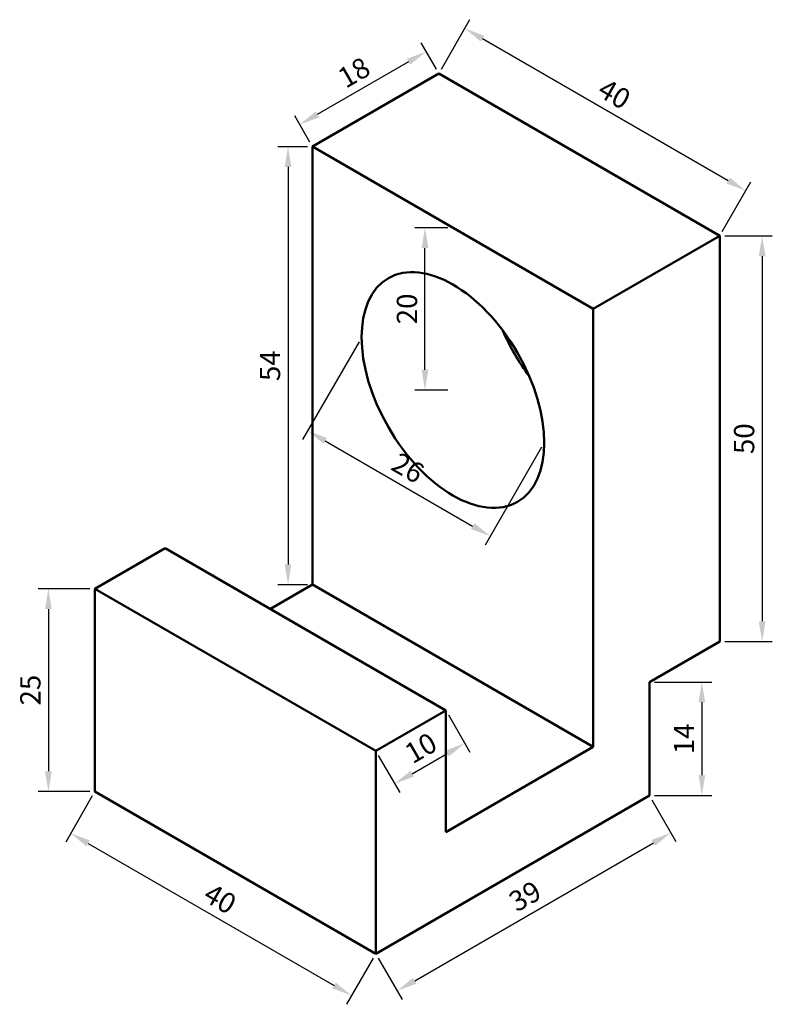
# Model space of a CAD drawing. Units: millimetres. Extents: x 3000 to 3093, y 728 to 849.
import ezdxf

# ---------------------------------------------------------------- set-up
doc = ezdxf.new("R2010")
doc.units = ezdxf.units.MM
doc.layers.add('M-DIMS', color=2, linetype='Continuous', lineweight=25)
doc.layers.add('M-OUTL', color=7, linetype='Continuous', lineweight=50)
doc.styles.get("Standard").update_dxf_attribs({"font": 'arial.ttf'})
doc.dimstyles.new('ISO-25', dxfattribs={"dimtxt": 2.5, "dimasz": 2.5, "dimexe": 1.25, "dimexo": 0.625, "dimtad": 1, "dimtxsty": 'Standard', "dimcen": 2.5, "dimadec": 0, "dimazin": 0, "dimtfac": 1, "dimtmove": 0, "dimatfit": 3, "dimfxl": 1, "dimarcsym": 0})

# ---------------------------------------------------------------- blocks, each defined once
blk = doc.blocks.new('*D1')
at = {"layer": 'Defpoints', "color": 0, "transparency": 16777216}
for p in [(3051.81, 842.52), (3089.67, 828.09), (3086.45, 822.52)]:
    blk.add_point(p, dxfattribs=at)
at = {"layer": 'M-DIMS', "color": 0, "lineweight": -2, "transparency": 16777216}
for p, q in [((3052.12, 843.06), (3055.65, 849.18)), ((3057.19, 846.84), (3087.5, 829.34)), ((3086.76, 823.06), (3090.29, 829.18))]:
    blk.add_line(p, q, dxfattribs=at)
at = {"layer": 'M-DIMS', "color": 0, "transparency": 16777216}
for points in [[(3057.4, 847.2), (3056.98, 846.48), (3055.03, 848.09)], [(3087.71, 829.7), (3087.3, 828.98), (3089.67, 828.09)]]:
    blk.add_solid(points, dxfattribs=at)
at = {"layer": 'M-DIMS', "color": 0, "transparency": 16777216, "insert": (3073.3, 839.74), "char_height": 2.5, "attachment_point": 5, "rotation": 330}
blk.add_mtext('40', dxfattribs=at)
blk = doc.blocks.new('*D2')
at = {"layer": 'Defpoints', "color": 0, "transparency": 16777216}
for p in [(3086.45, 822.52), (3086.45, 772.52), (3091.69, 772.52)]:
    blk.add_point(p, dxfattribs=at)
at = {"layer": 'M-DIMS', "color": 0, "lineweight": -2, "transparency": 16777216}
for p, q in [((3087.08, 822.52), (3092.94, 822.52)), ((3091.69, 820.02), (3091.69, 775.02)), ((3087.08, 772.52), (3092.94, 772.52))]:
    blk.add_line(p, q, dxfattribs=at)
at = {"layer": 'M-DIMS', "color": 0, "transparency": 16777216}
for points in [[(3091.27, 820.02), (3092.11, 820.02), (3091.69, 822.52)], [(3091.27, 775.02), (3092.11, 775.02), (3091.69, 772.52)]]:
    blk.add_solid(points, dxfattribs=at)
at = {"layer": 'M-DIMS', "color": 0, "transparency": 16777216, "insert": (3089.79, 797.52), "char_height": 2.5, "attachment_point": 5, "rotation": 90}
blk.add_mtext('50', dxfattribs=at)
blk = doc.blocks.new('*D3')
at = {"layer": 'Defpoints', "color": 0, "transparency": 16777216}
for p in [(3051.81, 842.52), (3034.65, 836.24), (3036.22, 833.52)]:
    blk.add_point(p, dxfattribs=at)
at = {"layer": 'M-DIMS', "color": 0, "lineweight": -2, "transparency": 16777216}
for p, q in [((3051.5, 843.06), (3049.62, 846.32)), ((3048.08, 843.99), (3036.82, 837.49)), ((3035.91, 834.06), (3034.03, 837.32))]:
    blk.add_line(p, q, dxfattribs=at)
at = {"layer": 'M-DIMS', "color": 0, "transparency": 16777216}
for points in [[(3047.87, 844.35), (3048.28, 843.63), (3050.24, 845.24)], [(3036.61, 837.85), (3037.03, 837.13), (3034.65, 836.24)]]:
    blk.add_solid(points, dxfattribs=at)
at = {"layer": 'M-DIMS', "color": 0, "transparency": 16777216, "insert": (3041.5, 842.39), "char_height": 2.5, "attachment_point": 5, "rotation": 30}
blk.add_mtext('18', dxfattribs=at)
blk = doc.blocks.new('*D4')
at = {"layer": 'Defpoints', "color": 0, "transparency": 16777216}
for p in [(3036.22, 833.52), (3033.21, 779.52), (3036.22, 779.52)]:
    blk.add_point(p, dxfattribs=at)
at = {"layer": 'M-DIMS', "color": 0, "lineweight": -2, "transparency": 16777216}
for p, q in [((3035.6, 833.52), (3031.96, 833.52)), ((3033.21, 831.02), (3033.21, 782.02)), ((3035.6, 779.52), (3031.96, 779.52))]:
    blk.add_line(p, q, dxfattribs=at)
at = {"layer": 'M-DIMS', "color": 0, "transparency": 16777216}
for points in [[(3032.79, 831.02), (3033.62, 831.02), (3033.21, 833.52)], [(3032.79, 782.02), (3033.62, 782.02), (3033.21, 779.52)]]:
    blk.add_solid(points, dxfattribs=at)
at = {"layer": 'M-DIMS', "color": 0, "transparency": 16777216, "insert": (3031.31, 806.52), "char_height": 2.5, "attachment_point": 5, "rotation": 90}
blk.add_mtext('54', dxfattribs=at)
blk = doc.blocks.new('*D5')
at = {"layer": 'Defpoints', "color": 0, "transparency": 16777216}
for p in [(3009.38, 779.02), (3003.65, 754.02), (3009.38, 754.02)]:
    blk.add_point(p, dxfattribs=at)
at = {"layer": 'M-DIMS', "color": 0, "lineweight": -2, "transparency": 16777216}
for p, q in [((3008.75, 779.02), (3002.4, 779.02)), ((3003.65, 776.52), (3003.65, 756.52)), ((3008.75, 754.02), (3002.4, 754.02))]:
    blk.add_line(p, q, dxfattribs=at)
at = {"layer": 'M-DIMS', "color": 0, "transparency": 16777216}
for points in [[(3003.23, 776.52), (3004.07, 776.52), (3003.65, 779.02)], [(3003.23, 756.52), (3004.07, 756.52), (3003.65, 754.02)]]:
    blk.add_solid(points, dxfattribs=at)
at = {"layer": 'M-DIMS', "color": 0, "transparency": 16777216, "insert": (3001.75, 766.52), "char_height": 2.5, "attachment_point": 5, "rotation": 90}
blk.add_mtext('25', dxfattribs=at)
blk = doc.blocks.new('*D6')
at = {"layer": 'Defpoints', "color": 0, "transparency": 16777216}
for p in [(3009.38, 754.02), (3044.02, 734.02), (3041.04, 728.87)]:
    blk.add_point(p, dxfattribs=at)
at = {"layer": 'M-DIMS', "color": 0, "lineweight": -2, "transparency": 16777216}
for p, q in [((3009.06, 753.48), (3005.78, 747.79)), ((3008.57, 747.62), (3038.88, 730.12)), ((3043.7, 733.48), (3040.42, 727.79))]:
    blk.add_line(p, q, dxfattribs=at)
at = {"layer": 'M-DIMS', "color": 0, "transparency": 16777216}
for points in [[(3008.77, 747.98), (3008.36, 747.26), (3006.4, 748.87)], [(3039.08, 730.48), (3038.67, 729.76), (3041.04, 728.87)]]:
    blk.add_solid(points, dxfattribs=at)
at = {"layer": 'M-DIMS', "color": 0, "transparency": 16777216, "insert": (3024.67, 740.52), "char_height": 2.5, "attachment_point": 5, "rotation": 330}
blk.add_mtext('40', dxfattribs=at)
blk = doc.blocks.new('*D7')
at = {"layer": 'Defpoints', "color": 0, "transparency": 16777216}
for p in [(3077.79, 753.52), (3080.44, 748.94), (3044.02, 734.02)]:
    blk.add_point(p, dxfattribs=at)
at = {"layer": 'M-DIMS', "color": 0, "lineweight": -2, "transparency": 16777216}
for p, q in [((3078.1, 752.98), (3081.06, 747.86)), ((3048.83, 730.69), (3078.27, 747.69)), ((3044.33, 733.48), (3047.29, 728.36))]:
    blk.add_line(p, q, dxfattribs=at)
at = {"layer": 'M-DIMS', "color": 0, "transparency": 16777216}
for points in [[(3078.06, 748.05), (3078.48, 747.33), (3080.44, 748.94)], [(3048.62, 731.05), (3049.04, 730.33), (3046.66, 729.44)]]:
    blk.add_solid(points, dxfattribs=at)
at = {"layer": 'M-DIMS', "color": 0, "transparency": 16777216, "insert": (3062.6, 740.84), "char_height": 2.5, "attachment_point": 5, "rotation": 30}
blk.add_mtext('39', dxfattribs=at)
blk = doc.blocks.new('*D8')
at = {"layer": 'Defpoints', "color": 0, "transparency": 16777216}
for p in [(3077.79, 767.52), (3077.79, 753.52), (3084.25, 753.52)]:
    blk.add_point(p, dxfattribs=at)
at = {"layer": 'M-DIMS', "color": 0, "lineweight": -2, "transparency": 16777216}
for p, q in [((3078.42, 767.52), (3085.5, 767.52)), ((3084.25, 765.02), (3084.25, 756.02)), ((3078.42, 753.52), (3085.5, 753.52))]:
    blk.add_line(p, q, dxfattribs=at)
at = {"layer": 'M-DIMS', "color": 0, "transparency": 16777216}
for points in [[(3083.84, 765.02), (3084.67, 765.02), (3084.25, 767.52)], [(3083.84, 756.02), (3084.67, 756.02), (3084.25, 753.52)]]:
    blk.add_solid(points, dxfattribs=at)
at = {"layer": 'M-DIMS', "color": 0, "transparency": 16777216, "insert": (3082.37, 760.52), "char_height": 2.5, "attachment_point": 5, "rotation": 90}
blk.add_mtext('14', dxfattribs=at)
blk = doc.blocks.new('*D9')
at = {"layer": 'Defpoints', "color": 0, "transparency": 16777216}
for p in [(3052.68, 764.02), (3055.02, 759.97), (3044.02, 759.02)]:
    blk.add_point(p, dxfattribs=at)
at = {"layer": 'M-DIMS', "color": 0, "lineweight": -2, "transparency": 16777216}
for p, q in [((3052.99, 763.48), (3055.64, 758.88)), ((3048.52, 756.22), (3052.85, 758.72)), ((3044.33, 758.48), (3046.98, 753.88))]:
    blk.add_line(p, q, dxfattribs=at)
at = {"layer": 'M-DIMS', "color": 0, "transparency": 16777216}
for points in [[(3052.65, 759.08), (3053.06, 758.36), (3055.02, 759.97)], [(3048.32, 756.58), (3048.73, 755.86), (3046.36, 754.97)]]:
    blk.add_solid(points, dxfattribs=at)
at = {"layer": 'M-DIMS', "color": 0, "transparency": 16777216, "insert": (3049.74, 759.11), "char_height": 2.5, "attachment_point": 5, "rotation": 30}
blk.add_mtext('10', dxfattribs=at)
blk = doc.blocks.new('*D10')
at = {"layer": 'Defpoints', "color": 0, "transparency": 16777216}
for p in [(3050.1, 823.52), (3053.54, 823.52), (3053.54, 803.52)]:
    blk.add_point(p, dxfattribs=at)
at = {"layer": 'M-DIMS', "color": 0, "lineweight": -2, "transparency": 16777216}
for p, q in [((3052.92, 823.52), (3048.85, 823.52)), ((3050.1, 806.02), (3050.1, 821.02)), ((3052.92, 803.52), (3048.85, 803.52))]:
    blk.add_line(p, q, dxfattribs=at)
at = {"layer": 'M-DIMS', "color": 0, "transparency": 16777216}
for points in [[(3049.69, 821.02), (3050.52, 821.02), (3050.1, 823.52)], [(3049.69, 806.02), (3050.52, 806.02), (3050.1, 803.52)]]:
    blk.add_solid(points, dxfattribs=at)
at = {"layer": 'M-DIMS', "color": 0, "transparency": 16777216, "insert": (3048.2, 813.52), "char_height": 2.5, "attachment_point": 5, "rotation": 90}
blk.add_mtext('20', dxfattribs=at)
blk = doc.blocks.new('*D11')
at = {"layer": 'Defpoints', "color": 0, "transparency": 16777216}
for p in [(3042.28, 810.02), (3064.8, 797.02), (3058.15, 785.5)]:
    blk.add_point(p, dxfattribs=at)
at = {"layer": 'M-DIMS', "color": 0, "lineweight": -2, "transparency": 16777216}
for p, q in [((3041.97, 809.48), (3035.01, 797.41)), ((3037.8, 797.25), (3055.98, 786.75)), ((3064.49, 796.48), (3057.52, 784.41))]:
    blk.add_line(p, q, dxfattribs=at)
at = {"layer": 'M-DIMS', "color": 0, "transparency": 16777216}
for points in [[(3038, 797.61), (3037.59, 796.89), (3035.63, 798.5)], [(3056.19, 787.11), (3055.77, 786.39), (3058.15, 785.5)]]:
    blk.add_solid(points, dxfattribs=at)
at = {"layer": 'M-DIMS', "color": 0, "transparency": 16777216, "insert": (3047.84, 793.64), "char_height": 2.5, "attachment_point": 5, "rotation": 330}
blk.add_mtext('26', dxfattribs=at)

msp = doc.modelspace()

# ---------------------------------------------------------------- linework, layer by layer
at = {"layer": 'M-OUTL'}
for p, q in [((3051.811, 842.522), (3036.223, 833.522)), ((3086.452, 822.522), (3051.811, 842.522)), ((3036.223, 833.522), (3070.864, 813.522)), ((3036.223, 833.522), (3036.223, 779.522)), ((3070.864, 813.522), (3086.452, 822.522)), ((3086.452, 772.522), (3086.452, 822.522)), ((3070.864, 813.522), (3070.864, 759.522)), ((3009.376, 779.022), (3018.036, 784.022)), ((3018.036, 784.022), (3052.677, 764.022)), ((3036.223, 779.522), (3031.027, 776.522)), ((3036.223, 779.522), (3070.864, 759.522)), ((3009.376, 754.022), (3009.376, 779.022)), ((3044.017, 759.022), (3009.376, 779.022)), ((3077.792, 767.522), (3086.452, 772.522)), ((3077.792, 753.522), (3077.792, 767.522)), ((3044.017, 759.022), (3052.677, 764.022)), ((3052.677, 749.022), (3052.677, 764.022)), ((3044.017, 759.022), (3044.017, 734.022)), ((3044.017, 734.022), (3044.017, 759.022)), ((3070.864, 759.522), (3052.677, 749.022)), ((3044.017, 734.022), (3009.376, 754.022)), ((3044.017, 734.022), (3077.792, 753.522))]:
    msp.add_line(p, q, dxfattribs=at)
msp.add_ellipse((3053.543, 803.522), major_axis=(7.961, -13.789), ratio=0.5773503, dxfattribs=at)
msp.add_ellipse((3069.132, 812.522), major_axis=(7.961, -13.789), ratio=0.5773503, start_param=4.5074378, end_param=4.9173401, dxfattribs=at)

# ---------------------------------------------------------------- dimensions: what is measured, and where the dimension line sits
at = {"layer": 'M-DIMS'}
for p1, p2, distance, picture, middle in [((3051.811, 842.522), (3086.452, 822.522), 6.432, '*D1', (3073.299, 839.74)), ((3051.811, 842.522), (3036.223, 833.522), -3.14, '*D3', (3041.496, 842.389)), ((3036.223, 833.522), (3036.223, 779.522), -3.015, '*D4', (3031.311, 806.522)), ((3053.543, 803.522), (3053.543, 823.522), 3.44, '*D10', (3048.202, 813.522)), ((3086.452, 822.522), (3086.452, 772.522), 5.239, '*D2', (3089.79, 797.522)), ((3042.285, 810.022), (3064.802, 797.022), -13.308, '*D11', (3047.84, 793.644)), ((3009.376, 779.022), (3009.376, 754.022), -5.726, '*D5', (3001.748, 766.522)), ((3077.792, 767.522), (3077.792, 753.522), 6.461, '*D8', (3082.373, 760.522)), ((3044.017, 759.022), (3052.677, 764.022), -4.683, '*D9', (3049.738, 759.114)), ((3009.376, 754.022), (3044.017, 734.022), -5.951, '*D6', (3024.672, 740.515)), ((3044.017, 734.022), (3077.792, 753.522), -5.29, '*D7', (3062.598, 740.839))]:
    dim = msp.add_aligned_dim(p1=p1, p2=p2, distance=distance, dimstyle='ISO-25', override={"dimclrd": 0, "dimclre": 0, "dimclrt": 0}, dxfattribs=at)
    dim.commit()
    dim.dimension.update_dxf_attribs({"geometry": picture, "text_midpoint": middle})

doc.saveas('drawing.dxf')
